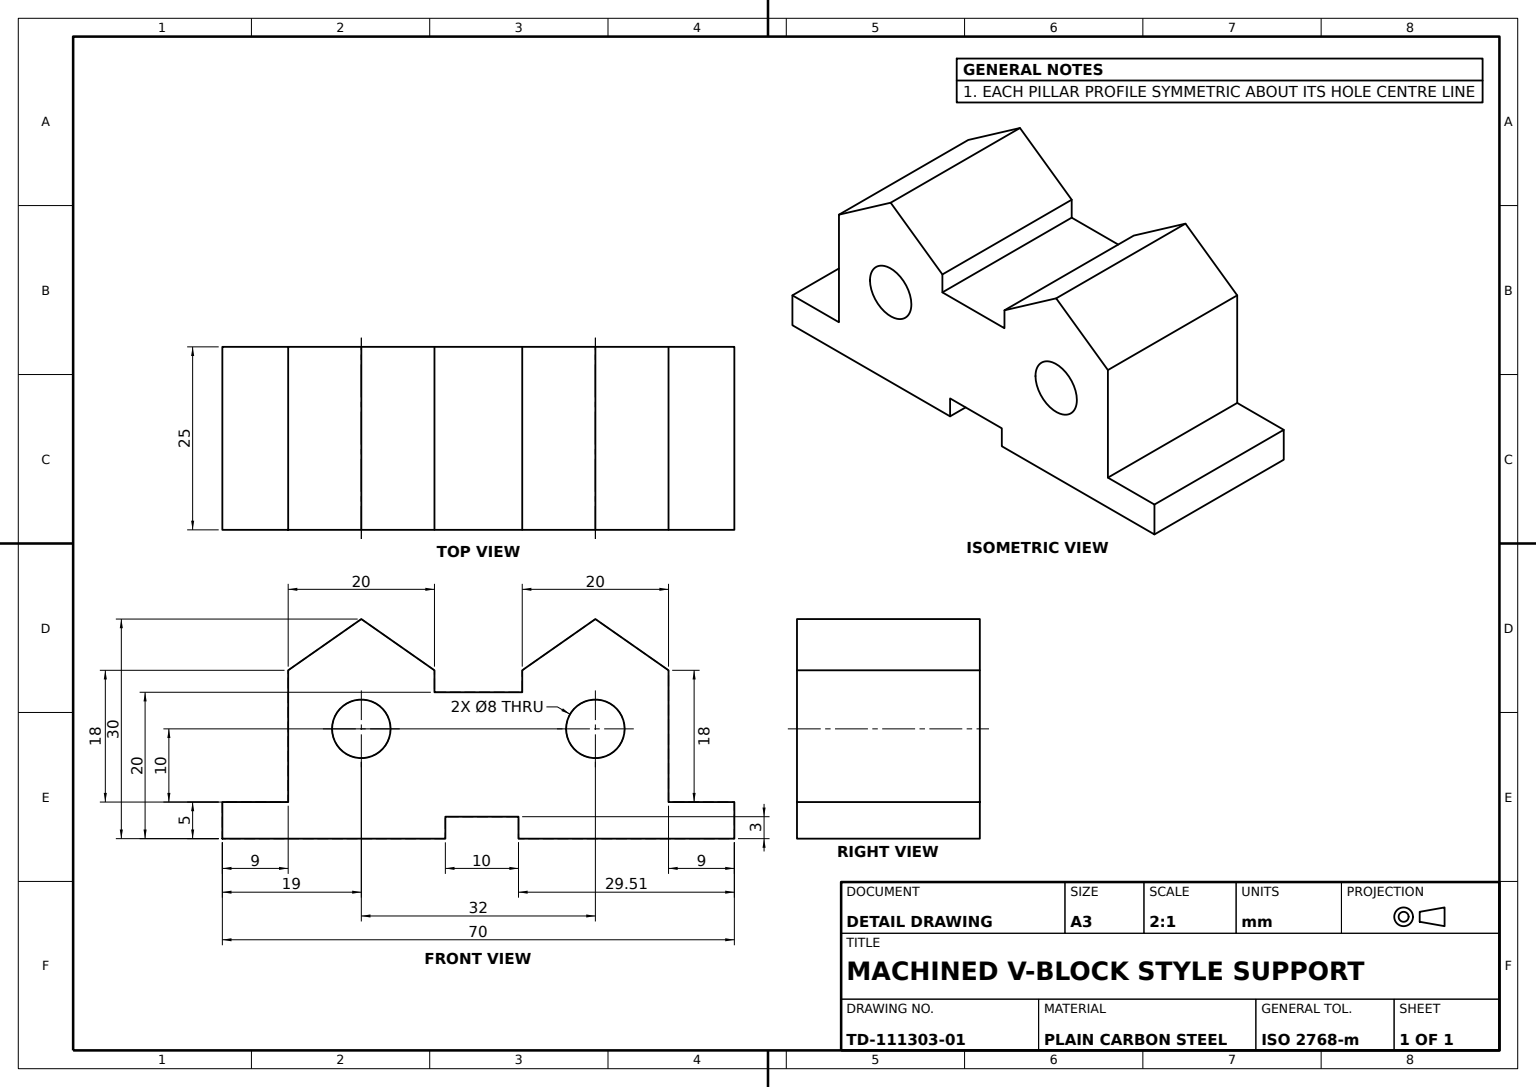
SolidWorks part; units mm, degrees
material "Plain Carbon Steel"
ref_plane "Front Plane" through (0, 0, 0) normal (0, 0, 1) x (1, 0, 0)
ref_plane "Top Plane" through (0, 0, 0) normal (0, 1, 0) x (1, 0, 0)
ref_plane "Right Plane" through (0, 0, 0) normal (1, 0, 0) x (0, 0, -1)
sketch "Base Plate Sketch" plane through (0, 0, 0) normal (0, 1, 0) x (1, 0, 0)
  line L0 (0, 0) -> (0, 25)
  line L1 (0, 25) -> (70, 25)
  line L2 (70, 25) -> (70, 0)
  line L3 (70, 0) -> (0, 0)
  dimension "D1" = 70
  dimension "D2" = 25
extrude "Base Plate 70x25x5" add sketch "Base Plate Sketch" along normal blind 5
sketch "Pillar Profile Sketch" plane through (0, 0, 0) normal (0, 0, 1) x (1, 0, 0)
  line L0 (9, 5) -> (9, 23)
  line L1 (0, 5) -> (70, 5) construction
  line L2 (9, 23) -> (19, 30)
  line L3 (19, 30) -> (29, 23)
  line L4 (29, 23) -> (29, 20)
  line L5 (29, 20) -> (41, 20)
  line L6 (41, 20) -> (41, 23)
  line L7 (41, 23) -> (51, 30)
  line L8 (51, 30) -> (61, 23)
  line L9 (61, 23) -> (61, 5)
  line L10 (61, 5) -> (9, 5)
  dimension "D1" = 9
  dimension "D2" = 9
  dimension "D3" = 25
  dimension "D4" = 25
  dimension "D5" = 18
  dimension "D6" = 18
  dimension "D7" = 10
  dimension "D8" = 10
  dimension "D9" = 10
  dimension "D10" = 10
  dimension "D11" = 3
  dimension "D12" = 3
extrude "Twin Pillars" add sketch "Pillar Profile Sketch" against normal blind 25
sketch "Cross Holes Sketch" plane through (0, 0, 0) normal (0, 0, 1) x (1, 0, 0)
  line L0 (61, 5) -> (61, 23) construction
  line L1 (9, 23) -> (9, 5) construction
  line L2 (0, 0) -> (70, 0) construction
  circle A0 centre (51, 15) radius 4
  circle A1 centre (19, 15) radius 4
  dimension "D1" = 8
  dimension "D2" = 8
  dimension "D3" = 10
  dimension "D4" = 10
  dimension "D5" = 15
  dimension "D6" = 15
extrude "Cross Holes 2xØ8" cut sketch "Cross Holes Sketch" against normal blind 35
sketch "Relief Slot Sketch" plane through (0, 0, 0) normal (0, 0, 1) x (1, 0, 0)
  line L0 (30.4887, 0) -> (30.4887, 3)
  line L1 (0, 0) -> (70, 0) construction
  line L2 (30.4887, 3) -> (40.4887, 3)
  line L3 (40.4887, 3) -> (40.4887, 0)
  line L4 (40.4887, 0) -> (30.4887, 0)
  line L5 (70, 5) -> (70, 0) construction
  dimension "D1" = 10
  dimension "D2" = 3
  dimension "D3" = 29.5113
extrude "Underside Relief Slot 10x3" cut sketch "Relief Slot Sketch" against normal blind 35
